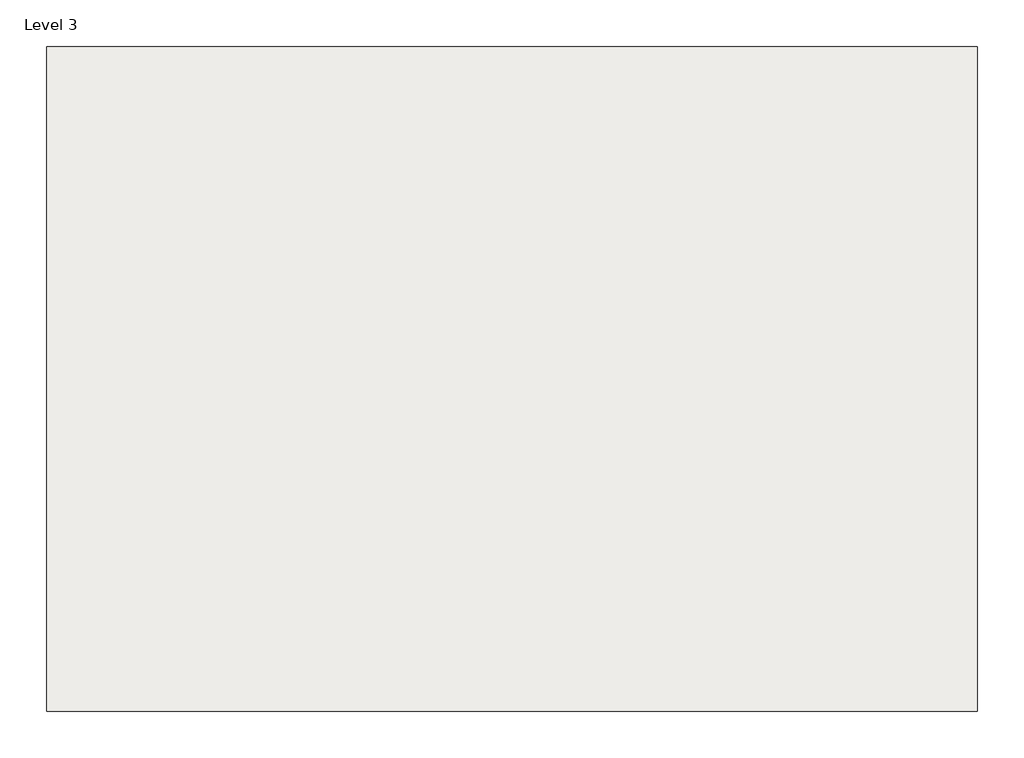
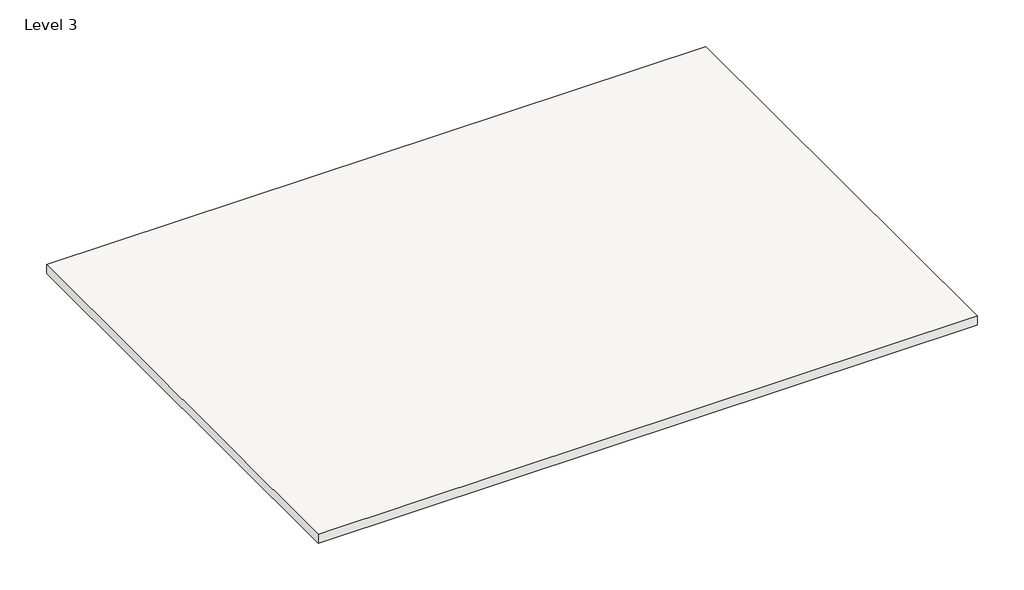
# One storey: 1 roof.
"""IFC4 building model written with IfcOpenShell, lengths in millimetres."""

from ifc_helpers import new_model, si_unit, frame, origin, place, context, project, spatial, polyline, outline, extrude, element, save

model = new_model("IFC4")

# Units and contexts
model_context = context("Model", 3, world=origin())
ifc_project = project(units=[si_unit("LENGTHUNIT", "METRE", prefix="MILLI")], contexts=[model_context])

# Site, building, storey
site = spatial("IfcSite", under=ifc_project)
building = spatial("IfcBuilding", under=site)
storey = spatial("IfcBuildingStorey", under=building, Name="Level 3", Elevation=6400.8)

# Roof
placement = place(None, origin())
element("IfcRoof", 1, ObjectType="Generic - 12\"", at=placement, inside=storey, context=model_context, shape_type="SweptSolid", body=[
    extrude(outline(polyline([(-14399.7415084, 8272.4935985), (6631.4584916, 8272.4935985), (6631.4584916, -6739.2866284), (-14399.7415084, -6739.2866284), (-14399.7415084, 8272.4935985)])), frame((0.0, 0.0, 6400.8), z_axis=(0.0, 0.0, 1.0), x_axis=(1.0, 0.0, 0.0)), (0.0, 0.0, 1.0), 304.8),
])

save(model, "model.ifc")

# Revit data of these elements
# Type "Generic - 12\""
#   Assembly Code = "B1020"
#   Layers, outside or top first: 1' - 0" no material (function 1)
# Element 1 (IfcRoof, "Generic - 12\"")
#   built-in parameter 1001705 = 22 (stored number, unit not read)
#   built-in parameter 1001710 = 33615
#   Phase Created = New Construction
#   Materials on its faces: "Default Roof"
# Materials
#   "Default Roof": colour RGB 88 101 114, transparency 0, Cost = 0
